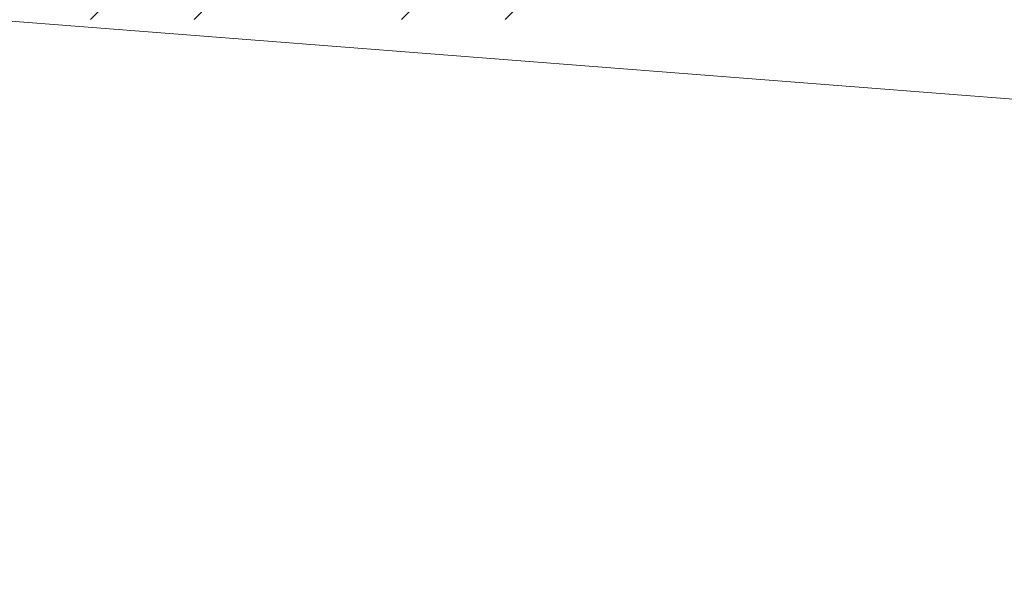
# Model space of a CAD drawing. Units: inches. Extents: x 1885 to 2748, y 783 to 2421.
# Tile 38 of 117: x 2013 to 2056, y 1534 to 1558. Entities that reach past the tile are written whole.
import ezdxf

# ---------------------------------------------------------------- set-up
doc = ezdxf.new("R2010")
doc.units = ezdxf.units.IN
doc.layers.add('A-FLOR-OPEN', color=8, linetype='Continuous', lineweight=13)
doc.layers.add('A-WALL-PATT', color=85, linetype='Continuous', lineweight=13, true_color=0x58ba48)

msp = doc.modelspace()

# ---------------------------------------------------------------- hatches: boundary and pattern name
at = {"layer": 'A-WALL-PATT'}
h = msp.add_hatch(dxfattribs=at)
h.set_pattern_fill('ANSI32', color=256)
h.paths.add_polyline_path([(2007.772, 2318.006), (1980.774, 2318.006), (1980.774, 2281.215), (1985.274, 2281.215), (1985.274, 2313.506), (2007.772, 2313.506), (2007.772, 2315.756)])
h.paths.add_polyline_path([(2094.324, 2318.006), (2067.772, 2318.006), (2067.772, 2313.506), (2094.324, 2313.506), (2094.324, 2315.756)])
h.paths.add_polyline_path([(2131.367, 2315.756), (2131.367, 2318.006), (2131.189, 2318.006), (2112.609, 2318.006), (2112.609, 2313.506), (2117.274, 2313.506), (2117.274, 2255.201), (2121.774, 2255.201), (2121.774, 2313.506), (2131.367, 2313.506)])
h.paths.add_polyline_path([(2190.512, 2318.006), (2155.367, 2318.006), (2155.367, 2313.506), (2169.774, 2313.506), (2169.774, 2229.506), (2121.774, 2229.506), (2121.774, 2233.451), (2119.524, 2233.451), (2117.274, 2233.451), (2117.274, 2201.101), (2121.774, 2201.101), (2121.774, 2225.006), (2169.774, 2225.006), (2169.774, 2165.006), (2306.274, 2165.006), (2306.274, 2066.006), (2310.774, 2066.006), (2344.274, 2066.006), (2486.274, 2066.006), (2486.274, 1886.006), (2483.02, 1886.006), (2483.02, 1881.506), (2486.274, 1881.506), (2486.274, 1880.678), (2490.774, 1880.678), (2490.774, 2070.506), (2344.274, 2070.506), (2310.774, 2070.506), (2310.774, 2165.006), (2310.774, 2173.636), (2308.524, 2173.636), (2306.274, 2173.636), (2306.274, 2169.506), (2174.274, 2169.506), (2174.274, 2313.506), (2190.512, 2313.506), (2190.512, 2315.756)])
h.paths.add_polyline_path([(1985.274, 2221.215), (1980.774, 2221.215), (1980.774, 2165.006), (1992.774, 2165.006), (1992.774, 2141.927), (1997.274, 2141.927), (1997.274, 2165.006), (2117.274, 2165.006), (2117.274, 2163.126), (2121.774, 2163.126), (2121.774, 2172.734), (2119.524, 2172.734), (2117.274, 2172.734), (2117.274, 2169.506), (1985.274, 2169.506)])
h.paths.add_polyline_path([(1997.274, 2105.927), (1992.774, 2105.927), (1992.774, 2070.506), (2016.774, 2070.506), (2016.774, 2059.123), (2019.024, 2059.123), (2021.274, 2059.123), (2021.274, 2070.506), (2117.274, 2070.506), (2117.274, 2022.506), (2114.423, 2022.506), (2114.423, 2018.006), (2123.627, 2018.006), (2123.627, 2020.256), (2123.627, 2022.506), (2121.774, 2022.506), (2121.774, 2142.587), (2119.524, 2142.587), (2117.274, 2142.587), (2117.274, 2075.006), (1997.274, 2075.006)])
h.paths.add_polyline_path([(2092.029, 2020.256), (2092.029, 2022.506), (2021.274, 2022.506), (2021.274, 2035.123), (2016.774, 2035.123), (2016.774, 2018.006), (2016.774, 1978.784), (2021.274, 1978.784), (2021.274, 2018.006), (2092.029, 2018.006)])
h.paths.add_polyline_path([(2260.938, 2022.506), (2153.105, 2022.506), (2153.105, 2020.256), (2153.105, 2018.006), (2155.274, 2018.006), (2155.274, 1886.006), (2107.629, 1886.006), (2107.629, 1881.506), (2182.911, 1881.506), (2182.911, 1883.756), (2182.911, 1886.006), (2159.774, 1886.006), (2159.774, 2018.006), (2260.938, 2018.006), (2260.938, 2020.256)])
h.paths.add_polyline_path([(2047.629, 1883.756), (2047.629, 1886.006), (2021.274, 1886.006), (2021.274, 1918.784), (2019.024, 1918.784), (2016.774, 1918.784), (2016.774, 1881.506), (2047.629, 1881.506)])
h.paths.add_polyline_path([(2306.361, 1883.756), (2306.361, 1886.006), (2296.274, 1886.006), (2296.274, 1982.006), (2316.535, 1982.006), (2316.535, 1984.256), (2316.535, 1986.506), (2296.274, 1986.506), (2296.274, 2022.506), (2289.276, 2022.506), (2289.276, 2018.006), (2291.774, 2018.006), (2291.774, 1886.006), (2242.911, 1886.006), (2242.911, 1881.506), (2306.361, 1881.506)], flags=17)
h.paths.add_polyline_path([(1985.274, 1843.006), (2021.6, 1843.006), (2021.534, 1845.441), (2021.477, 1847.506), (1980.774, 1847.506), (1980.774, 1809.446), (1985.274, 1809.446)])
h.paths.add_polyline_path([(2131.482, 1845.256), (2131.482, 1847.506), (2081.534, 1847.506), (2081.534, 1843.006), (2117.274, 1843.006), (2117.274, 1784.147), (2119.524, 1784.147), (2121.774, 1784.147), (2121.774, 1843.006), (2131.482, 1843.006)])
h.paths.add_polyline_path([(2203.886, 1847.506), (2155.482, 1847.506), (2155.482, 1843.006), (2169.774, 1843.006), (2169.774, 1759.006), (2121.774, 1759.006), (2121.774, 1761.457), (2117.274, 1761.457), (2117.274, 1730.429), (2121.774, 1730.429), (2121.774, 1754.506), (2177.421, 1754.506), (2177.421, 1756.756), (2177.421, 1759.006), (2174.274, 1759.006), (2174.274, 1843.006), (2203.886, 1843.006)])
h.paths.add_polyline_path([(2335.554, 1845.256), (2335.554, 1847.506), (2239.886, 1847.506), (2239.886, 1843.006), (2306.274, 1843.006), (2306.274, 1759.006), (2199.486, 1759.006), (2199.486, 1754.506), (2310.774, 1754.506), (2310.774, 1843.006), (2335.554, 1843.006)])
h.paths.add_polyline_path([(2348.774, 2022.506), (2344.274, 2022.506), (2344.274, 1986.506), (2341.681, 1986.506), (2341.681, 1982.006), (2344.274, 1982.006), (2344.274, 1886.006), (2330.361, 1886.006), (2330.361, 1881.506), (2361.627, 1881.506), (2361.627, 1883.756), (2361.627, 1886.006), (2348.774, 1886.006)], flags=17)
h.paths.add_polyline_path([(2283.251, 2315.756), (2283.251, 2318.006), (2238.512, 2318.006), (2238.512, 2313.506), (2283.251, 2313.506)], flags=17)
h.paths.add_polyline_path([(2363.274, 2348.006), (2388.677, 2348.006), (2388.677, 2350.256), (2388.677, 2352.506), (2358.774, 2352.506), (2358.774, 2348.006), (2358.774, 2318.006), (2344.481, 2318.006), (2344.481, 2313.506), (2358.774, 2313.506), (2358.774, 2229.506), (2310.774, 2229.506), (2310.774, 2231.952), (2306.274, 2231.952), (2306.274, 2205.611), (2310.774, 2205.611), (2310.774, 2225.006), (2358.774, 2225.006), (2358.774, 2211.506), (2452.329, 2211.506), (2452.329, 2213.756), (2452.329, 2216.006), (2363.274, 2216.006), (2363.274, 2318.006)])
h.paths.add_polyline_path([(2310.774, 2313.506), (2320.481, 2313.506), (2320.481, 2315.756), (2320.481, 2318.006), (2302.728, 2318.006), (2302.728, 2313.506), (2306.274, 2313.506), (2306.274, 2251.076), (2310.774, 2251.076)], flags=17)
h.paths.add_polyline_path([(2490.774, 2352.506), (2486.274, 2352.506), (2448.677, 2352.506), (2448.677, 2348.006), (2486.274, 2348.006), (2486.274, 2318.006), (2486.274, 2216.006), (2481.78, 2216.006), (2481.78, 2211.506), (2486.274, 2211.506), (2486.274, 2165.006), (2493.289, 2165.006), (2493.289, 2167.256), (2493.289, 2169.506), (2490.774, 2169.506), (2490.774, 2313.506), (2494.429, 2313.506), (2494.429, 2318.006), (2490.774, 2318.006)])
h.paths.add_polyline_path([(2534.653, 2318.006), (2515.691, 2318.006), (2515.691, 2313.506), (2534.653, 2313.506), (2534.653, 2315.756)])
h.paths.add_polyline_path([(2618.274, 2318.006), (2594.653, 2318.006), (2594.653, 2313.506), (2613.774, 2313.506), (2613.774, 2281.706), (2618.274, 2281.706)])
h.paths.add_polyline_path([(2618.274, 2221.706), (2613.774, 2221.706), (2613.774, 2169.506), (2554.019, 2169.506), (2554.019, 2165.006), (2613.774, 2165.006), (2613.774, 2152.878), (2618.274, 2152.878)])
h.paths.add_polyline_path([(2618.274, 2128.878), (2616.024, 2128.878), (2613.774, 2128.878), (2613.774, 2117.006), (2529.774, 2117.006), (2529.774, 2165.006), (2532.848, 2165.006), (2532.848, 2169.506), (2522.867, 2169.506), (2522.867, 2165.006), (2525.274, 2165.006), (2525.274, 2117.006), (2525.274, 2112.506), (2525.274, 2108.576), (2529.774, 2108.576), (2529.774, 2112.506), (2613.774, 2112.506), (2613.774, 2080.19), (2618.274, 2080.19)])
h.paths.add_polyline_path([(2618.274, 2044.19), (2616.024, 2044.19), (2613.774, 2044.19), (2613.774, 2015.506), (2529.774, 2015.506), (2529.774, 2088.582), (2527.524, 2088.582), (2525.274, 2088.582), (2525.274, 2011.006), (2613.774, 2011.006), (2613.774, 1956.755), (2618.274, 1956.755)])
h.paths.add_polyline_path([(2618.274, 1881.506), (2618.274, 1896.755), (2613.774, 1896.755), (2613.774, 1881.506), (2613.774, 1847.506), (2592.715, 1847.506), (2592.715, 1843.006), (2613.774, 1843.006), (2613.774, 1765.006), (2613.774, 1760.506), (2609.621, 1760.506), (2609.621, 1756.006), (2613.774, 1756.006), (2613.774, 1660.006), (2608.544, 1660.006), (2608.544, 1655.506), (2613.774, 1655.506), (2613.774, 1508.158), (2618.274, 1508.158)])
h.paths.add_polyline_path([(2565.774, 1843.006), (2568.997, 1843.006), (2568.997, 1847.506), (2490.774, 1847.506), (2490.774, 1849.7), (2488.524, 1849.7), (2486.274, 1849.7), (2486.274, 1847.506), (2477.274, 1847.506), (2477.274, 1838.506), (2477.274, 1821.493), (2486.274, 1821.493), (2486.274, 1838.506), (2561.274, 1838.506), (2561.274, 1765.006), (2486.274, 1765.006), (2486.274, 1786.157), (2477.274, 1786.157), (2477.274, 1765.006), (2477.274, 1756.006), (2486.274, 1756.006), (2565.774, 1756.006), (2585.621, 1756.006), (2585.621, 1758.256), (2585.621, 1760.506), (2565.774, 1760.506), (2565.774, 1765.006)])
h.paths.add_polyline_path([(2486.274, 1651.006), (2561.274, 1651.006), (2561.274, 1567.006), (2486.274, 1567.006), (2486.274, 1591.321), (2477.274, 1591.321), (2477.274, 1567.006), (2477.274, 1558.006), (2477.274, 1555.439), (2481.774, 1555.439), (2481.774, 1558.006), (2568.653, 1558.006), (2568.653, 1560.256), (2568.653, 1562.506), (2565.774, 1562.506), (2565.774, 1655.506), (2584.544, 1655.506), (2584.544, 1657.756), (2584.544, 1660.006), (2565.774, 1660.006), (2486.274, 1660.006), (2477.274, 1660.006), (2477.274, 1651.006), (2477.274, 1632.989), (2486.274, 1632.989)])
h.paths.add_polyline_path([(2449.967, 1883.756), (2449.967, 1886.006), (2421.627, 1886.006), (2421.627, 1881.506), (2449.967, 1881.506)], flags=17)
h.paths.add_polyline_path([(2447.274, 1847.506), (2395.554, 1847.506), (2395.554, 1843.006), (2442.774, 1843.006), (2442.774, 1809.27), (2447.274, 1809.27)])
h.paths.add_polyline_path([(1985.274, 1749.446), (1980.774, 1749.446), (1980.774, 1694.504), (1985.274, 1694.504), (1985.274, 1694.506), (1986.897, 1694.506), (1986.897, 1697.78), (1986.897, 1699.006), (1985.274, 1699.006)])
h.paths.add_polyline_path([(2152.774, 1699.006), (2121.774, 1699.006), (2121.774, 1703.668), (2119.524, 1703.668), (2117.274, 1703.668), (2117.274, 1699.006), (2009.219, 1699.006), (2009.219, 1694.506), (2148.274, 1694.506), (2148.274, 1692.631), (2152.774, 1692.631)])
h.paths.add_polyline_path([(2016.274, 1694.506), (2011.774, 1694.506), (2011.774, 1558.006), (2040.806, 1558.006), (2040.806, 1560.256), (2040.806, 1562.506), (2016.274, 1562.506)])
h.paths.add_polyline_path([(2152.774, 1663.017), (2150.524, 1663.017), (2148.274, 1663.017), (2148.274, 1562.506), (2100.806, 1562.506), (2100.806, 1558.006), (2165.119, 1558.006), (2165.119, 1560.256), (2165.119, 1562.506), (2152.774, 1562.506), (2152.774, 1610.506), (2224.774, 1610.506), (2224.774, 1607.99), (2229.274, 1607.99), (2229.274, 1615.006), (2152.774, 1615.006)])
h.paths.add_polyline_path([(2238.613, 1560.256), (2238.613, 1562.506), (2229.274, 1562.506), (2229.274, 1588.756), (2227.024, 1588.763), (2224.774, 1588.771), (2224.774, 1562.506), (2189.119, 1562.506), (2189.119, 1558.006), (2238.613, 1558.006)])
h.paths.add_polyline_path([(2336.024, 1560.256), (2336.024, 1562.506), (2310.774, 1562.506), (2310.774, 1656.347), (2308.524, 1656.347), (2306.274, 1656.347), (2306.274, 1562.506), (2286.613, 1562.506), (2286.613, 1558.006), (2336.024, 1558.006)])
h.paths.add_polyline_path([(2447.274, 1690.968), (2445.024, 1690.968), (2442.774, 1690.968), (2442.774, 1687.006), (2306.274, 1687.006), (2306.274, 1680.75), (2310.774, 1680.75), (2310.774, 1682.506), (2442.774, 1682.506), (2442.774, 1562.506), (2396.024, 1562.506), (2396.024, 1558.006), (2447.274, 1558.006)])
h.paths.add_polyline_path([(2447.274, 1749.27), (2445.024, 1749.27), (2442.774, 1749.27), (2442.774, 1717.232), (2447.274, 1717.232)])
h.paths.add_polyline_path([(2044.674, 1521.756), (2044.674, 1524.006), (2007.274, 1524.006), (2007.274, 1503.49), (2009.524, 1503.49), (2011.774, 1503.49), (2011.774, 1519.506), (2044.674, 1519.506)])
h.paths.add_polyline_path([(2177.969, 1521.756), (2177.969, 1524.006), (2104.674, 1524.006), (2104.674, 1519.506), (2145.774, 1519.506), (2145.774, 1387.506), (2143.37, 1387.506), (2143.37, 1383.006), (2251.585, 1383.006), (2251.585, 1385.256), (2251.585, 1387.506), (2150.274, 1387.506), (2150.274, 1519.506), (2177.969, 1519.506)])
h.paths.add_polyline_path([(2298.704, 1524.006), (2237.969, 1524.006), (2237.969, 1519.506), (2282.274, 1519.506), (2282.274, 1387.506), (2279.683, 1387.506), (2279.683, 1383.006), (2286.774, 1383.006), (2286.774, 1419.006), (2312.451, 1419.006), (2312.451, 1421.256), (2312.451, 1423.506), (2286.774, 1423.506), (2286.774, 1519.506), (2298.704, 1519.506), (2298.704, 1521.722)], flags=17)
h.paths.add_polyline_path([(2361.897, 1521.756), (2361.897, 1524.006), (2322.704, 1524.006), (2322.704, 1519.506), (2334.774, 1519.506), (2334.774, 1423.506), (2331.93, 1423.506), (2331.93, 1419.006), (2334.774, 1419.006), (2334.774, 1387.506), (2334.774, 1383.228), (2339.274, 1383.228), (2339.274, 1387.506), (2339.274, 1519.506), (2361.897, 1519.506)], flags=17)
h.paths.add_polyline_path([(2447.274, 1521.756), (2447.274, 1524.006), (2421.897, 1524.006), (2421.897, 1519.506), (2447.274, 1519.506)], flags=17)
h.paths.add_polyline_path([(2481.774, 1529.6), (2479.524, 1529.6), (2477.274, 1529.6), (2477.274, 1524.006), (2474.489, 1524.006), (2474.489, 1519.506), (2477.274, 1519.506), (2477.274, 1334.506), (2296.774, 1334.506), (2296.774, 1240.506), (2160.274, 1240.506), (2160.274, 1180.506), (2112.274, 1180.506), (2112.274, 1207.692), (2110.024, 1207.692), (2107.774, 1207.692), (2107.774, 1171.609), (2112.274, 1171.609), (2112.274, 1176.006), (2160.274, 1176.006), (2160.274, 1092.006), (2144.221, 1092.006), (2144.221, 1087.506), (2189.497, 1087.506), (2189.497, 1089.756), (2189.497, 1092.006), (2164.774, 1092.006), (2164.774, 1236.006), (2296.774, 1236.006), (2296.774, 1231.912), (2301.274, 1231.912), (2301.274, 1330.006), (2481.774, 1330.006), (2481.774, 1387.506)])
h.paths.add_polyline_path([(2618.274, 1448.158), (2613.774, 1448.158), (2613.774, 1382.506), (2529.774, 1382.506), (2525.274, 1382.506), (2525.274, 1307.062), (2529.774, 1307.062), (2529.774, 1378.006), (2613.774, 1378.006), (2613.774, 1354.988), (2618.274, 1354.988)])
h.paths.add_polyline_path([(2618.274, 1318.988), (2613.774, 1318.988), (2613.774, 1281.006), (2529.774, 1281.006), (2529.774, 1283.786), (2527.524, 1283.786), (2525.274, 1283.786), (2525.274, 1228.506), (2516.794, 1228.506), (2516.794, 1224.006), (2533.484, 1224.006), (2533.484, 1226.256), (2533.484, 1228.506), (2529.774, 1228.506), (2529.774, 1276.506), (2613.774, 1276.506), (2613.774, 1266.02), (2618.274, 1266.02)])
h.paths.add_polyline_path([(2618.274, 1134.964), (2613.774, 1134.964), (2613.774, 1092.006), (2594.545, 1092.006), (2594.545, 1087.506), (2618.274, 1087.506)])
h.paths.add_polyline_path([(2534.545, 1092.006), (2509.765, 1092.006), (2509.765, 1087.506), (2534.545, 1087.506), (2534.545, 1089.756)])
h.paths.add_polyline_path([(2481.274, 1224.006), (2484.117, 1224.006), (2484.117, 1226.256), (2484.117, 1228.506), (2476.774, 1228.506), (2476.774, 1198.506), (2471.61, 1198.506), (2471.61, 1194.006), (2476.774, 1194.006), (2476.774, 1062.006), (2436.894, 1062.006), (2436.894, 1057.506), (2476.774, 1057.506), (2481.274, 1057.506), (2481.274, 1062.006), (2481.274, 1087.506), (2485.354, 1087.506), (2485.354, 1089.756), (2485.354, 1092.006), (2481.274, 1092.006), (2481.274, 1117.506)])
h.paths.add_polyline_path([(2439.898, 1198.506), (2349.274, 1198.506), (2349.274, 1194.006), (2349.274, 1180.506), (2301.274, 1180.506), (2301.274, 1201.896), (2299.024, 1201.896), (2296.774, 1201.896), (2296.774, 1172.335), (2299.024, 1172.335), (2301.274, 1172.335), (2301.274, 1176.006), (2349.274, 1176.006), (2349.274, 1092.006), (2334.452, 1092.006), (2334.452, 1087.506), (2349.274, 1087.506), (2349.274, 1057.506), (2353.774, 1057.506), (2376.894, 1057.506), (2376.894, 1059.756), (2376.894, 1062.006), (2353.774, 1062.006), (2353.774, 1087.506), (2353.774, 1180.506), (2353.774, 1194.006), (2439.898, 1194.006), (2439.898, 1196.256)])
h.paths.add_polyline_path([(2270.596, 1089.756), (2270.596, 1092.006), (2249.497, 1092.006), (2249.497, 1087.506), (2270.596, 1087.506)], flags=17)
h.paths.add_polyline_path([(2310.452, 1092.006), (2301.274, 1092.006), (2301.274, 1153.292), (2296.774, 1153.292), (2296.774, 1092.006), (2293.786, 1092.006), (2293.786, 1087.506), (2310.452, 1087.506), (2310.452, 1089.756)], flags=17)
h.paths.add_polyline_path([(2112.274, 1150.328), (2110.024, 1150.328), (2107.774, 1150.328), (2107.774, 1092.006), (2104.465, 1092.006), (2104.465, 1087.506), (2120.221, 1087.506), (2120.221, 1089.756), (2120.221, 1092.006), (2112.274, 1092.006)])
h.paths.add_polyline_path([(2082.172, 1092.006), (2058.144, 1092.006), (2058.144, 1087.506), (2082.172, 1087.506), (2082.172, 1089.756)])
h.paths.add_polyline_path([(1975.774, 1145.638), (1971.274, 1145.638), (1971.274, 1087.506), (1980.774, 1087.506), (1998.144, 1087.506), (1998.144, 1089.756), (1998.144, 1092.006), (1985.274, 1092.006), (1975.774, 1092.006)])
h.paths.add_polyline_path([(2112.274, 1244.385), (2110.024, 1244.385), (2107.774, 1244.385), (2107.774, 1240.506), (1992.274, 1240.506), (1992.274, 1271.008), (1987.774, 1271.008), (1987.774, 1240.506), (1980.774, 1240.506), (1975.774, 1240.506), (1971.274, 1240.506), (1971.274, 1205.638), (1975.774, 1205.638), (1975.774, 1236.006), (2107.774, 1236.006), (2107.774, 1233.444), (2112.274, 1233.444), (2112.274, 1236.006)])
h.paths.add_polyline_path([(2112.274, 1383.006), (2114.783, 1383.006), (2114.783, 1385.256), (2114.783, 1387.506), (2102.476, 1387.506), (2102.476, 1383.006), (2107.774, 1383.006), (2107.774, 1335.006), (2011.774, 1335.006), (2011.774, 1349.939), (2007.274, 1349.939), (2007.274, 1335.006), (1987.774, 1335.006), (1987.774, 1330.506), (1987.774, 1307.008), (1992.274, 1307.008), (1992.274, 1330.506), (2007.274, 1330.506), (2107.774, 1330.506), (2107.774, 1264.711), (2112.274, 1264.711)])
h.paths.add_polyline_path([(2077.857, 1387.506), (2011.774, 1387.506), (2011.774, 1390.036), (2009.524, 1390.036), (2007.274, 1390.036), (2007.274, 1373.939), (2011.774, 1373.939), (2011.774, 1383.006), (2077.857, 1383.006)])
h.paths.add_polyline_path([(2011.774, 1443.49), (2007.274, 1443.49), (2007.274, 1410.248), (2011.774, 1410.248)])

# ---------------------------------------------------------------- linework, layer by layer
at = {"layer": 'A-FLOR-OPEN'}
msp.add_line((2447.274, 1524.006), (2011.774, 1558.006), dxfattribs=at)

doc.saveas('drawing.dxf')
